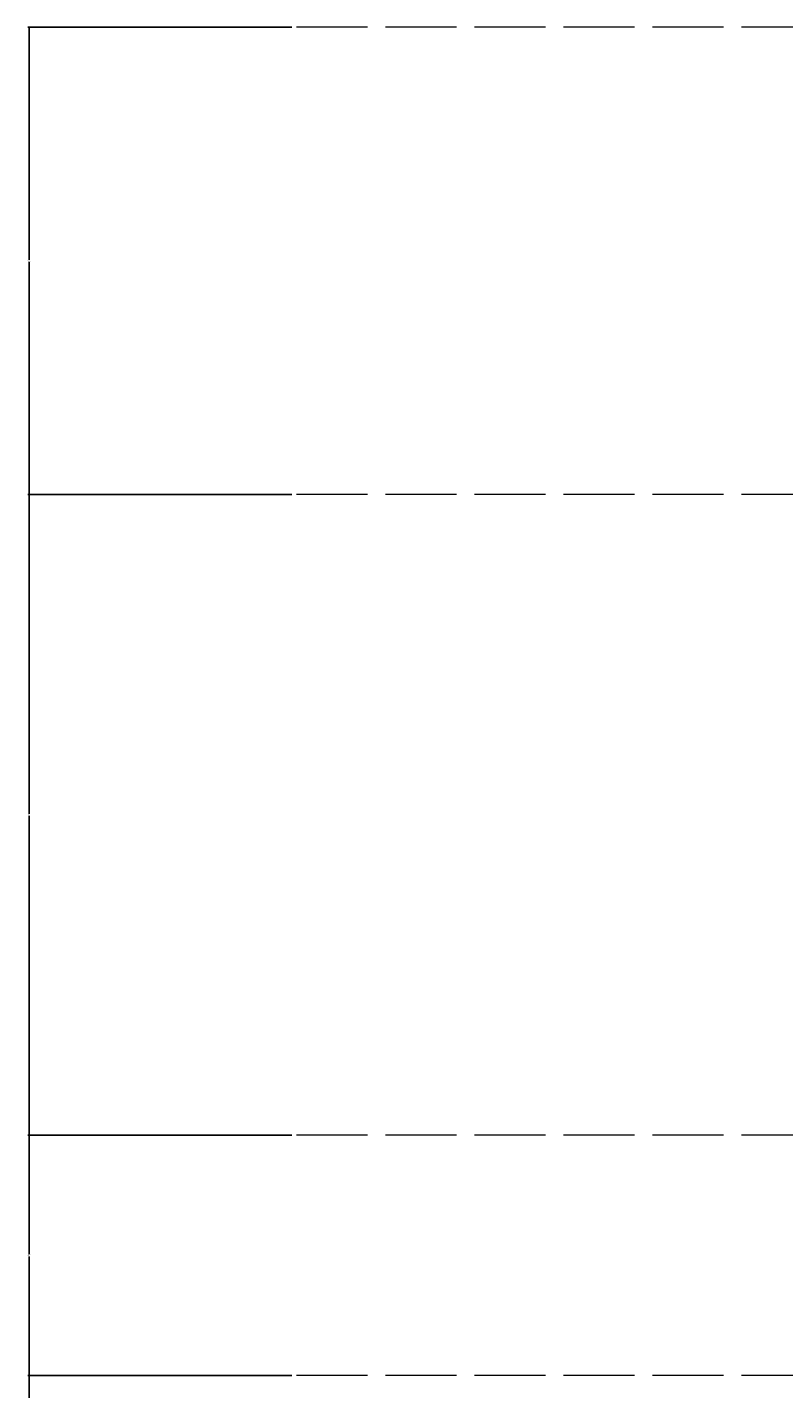
# Model space of a CAD drawing. Units: inches. Extents: x 1159 to 4240, y 1112 to 2085.
# Tile 5 of 13: x 1159 to 1286, y 1734 to 1963. Entities that reach past the tile are written whole.
import ezdxf

# ---------------------------------------------------------------- set-up
doc = ezdxf.new("R2010")
doc.units = ezdxf.units.IN
doc.linetypes.add('ACAD_ISO02W100', pattern=[15, 12, -3])
doc.layers.add('A-ANNO-DIMS', color=2, linetype='Continuous', lineweight=18)
doc.layers.add('A-GRID', color=8, linetype='ACAD_ISO02W100', lineweight=13)
doc.styles.get("Standard").update_dxf_attribs({"font": 'arial.ttf'})
doc.dimstyles.get("Standard").update_dxf_attribs({"dimtxt": 0.18, "dimasz": 0.18, "dimexe": 0.18, "dimexo": 0.0625, "dimgap": 0.09, "dimtad": 0, "dimtih": 1, "dimtoh": 1, "dimdec": 4, "dimzin": 0, "dimdsep": 46, "dimtxsty": 'Standard', "dimcen": 0.09, "dimadec": 0, "dimazin": 0, "dimtfac": 1, "dimtdec": 4, "dimtofl": 0, "dimtmove": 0, "dimatfit": 3, "dimfxl": 1, "dimtolj": 1, "dimtzin": 0, "dimarcsym": 0})

# ---------------------------------------------------------------- blocks, each defined once
blk = doc.blocks.new('HOUSE-35x60-SETTING-OUT-GRID')
for p, q in [((582.7, 806.25), (0, 806.25)), ((582.7, 727.5), (0, 727.5)), ((582.7, 619.5), (0, 619.5)), ((582.7, 579), (0, 579))]:
    blk.add_line(p, q)
blk = doc.blocks.new('*D42')
at = {"layer": 'A-ANNO-DIMS', "color": 0, "lineweight": -2, "transparency": 16777216}
for p, q in [((1203.25, 1735.95), (1158.78, 1735.95)), ((1158.96, 1735.77), (1158.96, 1703.88)), ((1158.96, 1671.63), (1158.96, 1703.52)), ((1203.25, 1671.45), (1158.78, 1671.45))]:
    blk.add_line(p, q, dxfattribs=at)
at = {"layer": 'A-ANNO-DIMS', "color": 0, "lineweight": 100, "transparency": 16777216}
for points in [[(1158.93, 1735.77), (1158.99, 1735.77), (1158.96, 1735.95)], [(1158.93, 1671.63), (1158.99, 1671.63), (1158.96, 1671.45)]]:
    blk.add_solid(points, dxfattribs=at)
at = {"layer": 'Defpoints', "color": 0, "lineweight": 100, "transparency": 16777216}
for p in [(1158.96, 1735.95), (1203.31, 1735.95), (1203.31, 1671.45)]:
    blk.add_point(p, dxfattribs=at)
at = {"layer": 'A-ANNO-DIMS', "color": 0, "transparency": 16777216, "insert": (1158.96, 1703.7), "char_height": 0.18, "attachment_point": 5}
blk.add_mtext('\\A1;64.5', dxfattribs=at)
blk = doc.blocks.new('*D43')
at = {"layer": 'A-ANNO-DIMS', "color": 0, "lineweight": -2, "transparency": 16777216}
for p, q in [((1203.25, 1776.45), (1158.78, 1776.45)), ((1158.96, 1776.27), (1158.96, 1756.38)), ((1158.96, 1736.13), (1158.96, 1756.02)), ((1203.25, 1735.95), (1158.78, 1735.95))]:
    blk.add_line(p, q, dxfattribs=at)
at = {"layer": 'A-ANNO-DIMS', "color": 0, "lineweight": 100, "transparency": 16777216}
for points in [[(1158.93, 1776.27), (1158.99, 1776.27), (1158.96, 1776.45)], [(1158.93, 1736.13), (1158.99, 1736.13), (1158.96, 1735.95)]]:
    blk.add_solid(points, dxfattribs=at)
at = {"layer": 'Defpoints', "color": 0, "lineweight": 100, "transparency": 16777216}
for p in [(1158.96, 1776.45), (1203.31, 1776.45), (1203.31, 1735.95)]:
    blk.add_point(p, dxfattribs=at)
at = {"layer": 'A-ANNO-DIMS', "color": 0, "transparency": 16777216, "insert": (1158.96, 1756.2), "char_height": 0.18, "attachment_point": 5}
blk.add_mtext('\\A1;40.5', dxfattribs=at)
blk = doc.blocks.new('*D44')
at = {"layer": 'A-ANNO-DIMS', "color": 0, "lineweight": -2, "transparency": 16777216}
for p, q in [((1203.25, 1884.45), (1158.78, 1884.45)), ((1158.96, 1884.27), (1158.96, 1830.63)), ((1158.96, 1776.63), (1158.96, 1830.27)), ((1203.25, 1776.45), (1158.78, 1776.45))]:
    blk.add_line(p, q, dxfattribs=at)
at = {"layer": 'A-ANNO-DIMS', "color": 0, "lineweight": 100, "transparency": 16777216}
for points in [[(1158.93, 1884.27), (1158.99, 1884.27), (1158.96, 1884.45)], [(1158.93, 1776.63), (1158.99, 1776.63), (1158.96, 1776.45)]]:
    blk.add_solid(points, dxfattribs=at)
at = {"layer": 'Defpoints', "color": 0, "lineweight": 100, "transparency": 16777216}
for p in [(1158.96, 1884.45), (1203.31, 1884.45), (1203.31, 1776.45)]:
    blk.add_point(p, dxfattribs=at)
at = {"layer": 'A-ANNO-DIMS', "color": 0, "transparency": 16777216, "insert": (1158.96, 1830.45), "char_height": 0.18, "attachment_point": 5}
blk.add_mtext('\\A1;108', dxfattribs=at)
blk = doc.blocks.new('*D45')
at = {"layer": 'A-ANNO-DIMS', "color": 0, "lineweight": -2, "transparency": 16777216}
for p, q in [((1203.25, 1963.2), (1158.78, 1963.2)), ((1158.96, 1963.02), (1158.96, 1924.01)), ((1158.96, 1884.63), (1158.96, 1923.65)), ((1203.25, 1884.45), (1158.78, 1884.45))]:
    blk.add_line(p, q, dxfattribs=at)
at = {"layer": 'A-ANNO-DIMS', "color": 0, "lineweight": 100, "transparency": 16777216}
for points in [[(1158.93, 1963.02), (1158.99, 1963.02), (1158.96, 1963.2)], [(1158.93, 1884.63), (1158.99, 1884.63), (1158.96, 1884.45)]]:
    blk.add_solid(points, dxfattribs=at)
at = {"layer": 'Defpoints', "color": 0, "lineweight": 100, "transparency": 16777216}
for p in [(1158.96, 1963.2), (1203.31, 1963.2), (1203.31, 1884.45)]:
    blk.add_point(p, dxfattribs=at)
at = {"layer": 'A-ANNO-DIMS', "color": 0, "transparency": 16777216, "insert": (1158.96, 1923.83), "char_height": 0.18, "attachment_point": 5}
blk.add_mtext('\\A1;78.75', dxfattribs=at)

msp = doc.modelspace()

# ---------------------------------------------------------------- block references
at = {"layer": 'A-GRID'}
msp.add_blockref('HOUSE-35x60-SETTING-OUT-GRID', (1203.31, 1156.954), dxfattribs=at)

# ---------------------------------------------------------------- dimensions: what is measured, and where the dimension line sits
at = {"layer": 'A-ANNO-DIMS'}
for base, p1, p2, override, picture, middle in [((1158.96, 1963.202), (1203.31, 1884.452), (1203.31, 1963.202), {"dimdec": 2, "dimlfac": 1, "dimrnd": 0, "dimzin": 0, "dimdsep": 46, "dimlunit": 2}, '*D45', (1158.96, 1923.827)), ((1158.96, 1884.452), (1203.31, 1776.452), (1203.31, 1884.452), {"dimdec": 0, "dimlfac": 1, "dimrnd": 0, "dimzin": 0, "dimdsep": 46, "dimlunit": 2}, '*D44', (1158.96, 1830.452)), ((1158.96, 1776.452), (1203.31, 1735.952), (1203.31, 1776.452), {"dimdec": 1, "dimlfac": 1, "dimrnd": 0, "dimzin": 0, "dimdsep": 46, "dimlunit": 2}, '*D43', (1158.96, 1756.202)), ((1158.96, 1735.952), (1203.31, 1671.452), (1203.31, 1735.952), {"dimdec": 1, "dimlfac": 1, "dimrnd": 0, "dimzin": 0, "dimdsep": 46, "dimlunit": 2}, '*D42', (1158.96, 1703.702))]:
    dim = msp.add_linear_dim(base=base, p1=p1, p2=p2, angle=90, dimstyle='Standard', override=override, dxfattribs=at)
    dim.commit()
    dim.dimension.update_dxf_attribs({"geometry": picture, "text_midpoint": middle})

doc.saveas('drawing.dxf')
